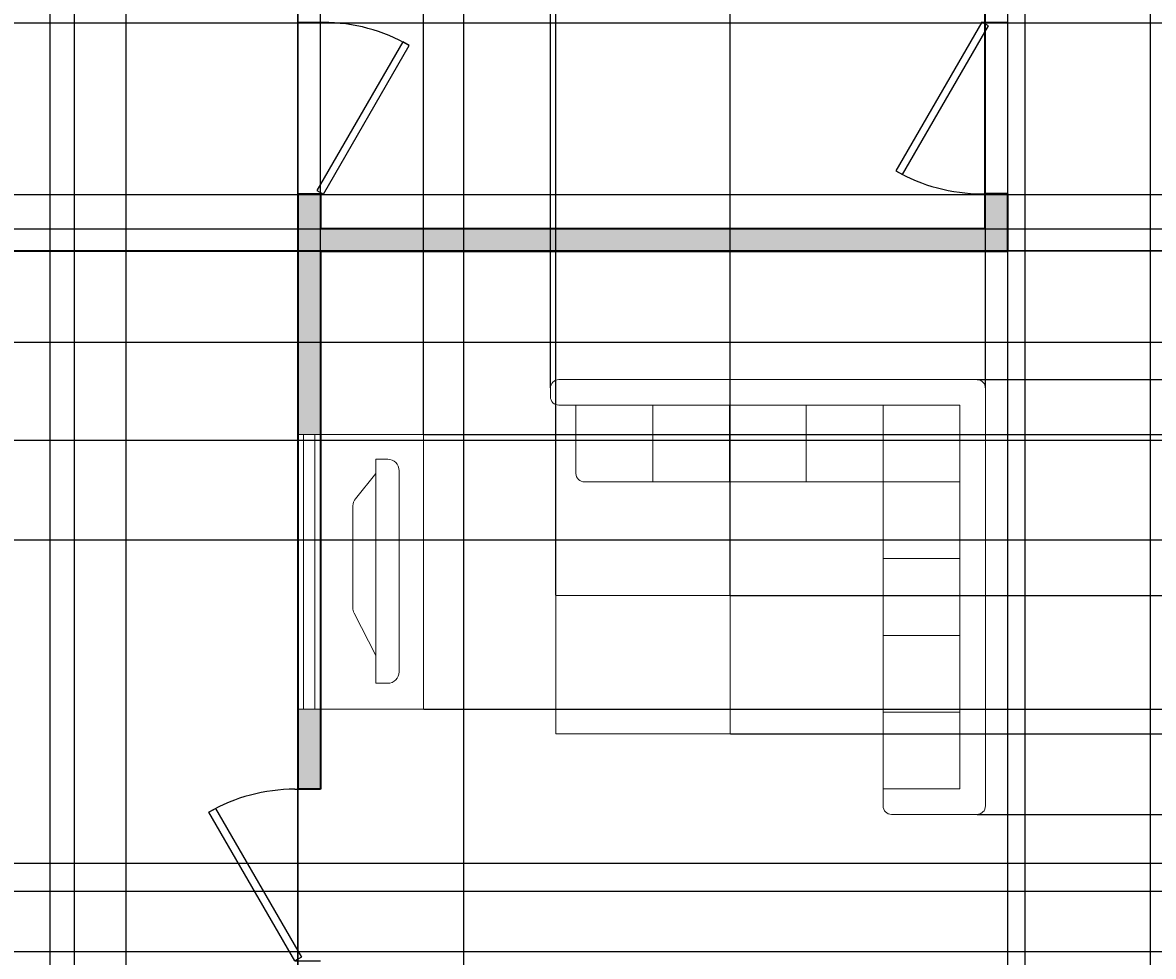
# Model space of a CAD drawing. Units: inches. Extents: x 1531 to 2263, y 2711 to 3216.
# Tile 5 of 12: x 1728 to 1925, y 2903 to 3066. Entities that reach past the tile are written whole.
import ezdxf

# ---------------------------------------------------------------- set-up
doc = ezdxf.new("R2010")
doc.units = ezdxf.units.IN
for name, color, linetype, lineweight in [('A-ANNO-DIMS', 2, 'Continuous', 18), ('A-DOOR', 3, 'Continuous', 25), ('A-EQPM', 8, 'Continuous', 18), ('A-FLOR-CASE', 9, 'Continuous', 18), ('A-FURN', 8, 'Continuous', 18), ('A-GLAZ', 4, 'Continuous', 18), ('A-WALL', 7, 'Continuous', 35)]:
    doc.layers.add(name, color=color, linetype=linetype, lineweight=lineweight)
doc.layers.add('A-WALL-PATT', color=18, linetype='Continuous', lineweight=13, true_color=0x000000)
doc.styles.get("Standard").update_dxf_attribs({"font": 'arial.ttf'})
doc.dimstyles.get("Standard").update_dxf_attribs({"dimtxt": 0.18, "dimasz": 0.18, "dimexe": 0.18, "dimexo": 0.0625, "dimgap": 0.09, "dimtad": 0, "dimtih": 1, "dimtoh": 1, "dimdec": 4, "dimzin": 0, "dimdsep": 46, "dimtxsty": 'Standard', "dimcen": 0.09, "dimadec": 0, "dimazin": 0, "dimtfac": 1, "dimtdec": 4, "dimtofl": 0, "dimtmove": 0, "dimatfit": 3, "dimfxl": 1, "dimtolj": 1, "dimtzin": 0, "dimarcsym": 0})

# ---------------------------------------------------------------- blocks, each defined once
blk = doc.blocks.new('*U5')
for p, q in [((0, 0), (0, -6)), ((-40, 0), (-40, -6))]:
    blk.add_line(p, q)
blk.add_lwpolyline([(0, 0), (-34.64, 20), (-35.52, 18.48), (-0.88, -1.52)], close=True)
blk.add_arc((0, 0), 40, 150, 180)
blk = doc.blocks.new('*U6')
for p, q in [((0, 0), (0, 6)), ((40, 0), (40, 6))]:
    blk.add_line(p, q)
blk.add_lwpolyline([(0, 0), (34.64, -20), (35.52, -18.48), (0.87, 1.52)], close=True)
blk.add_arc((0, 0), 40, 330, 0)
blk = doc.blocks.new('*U4')
for p, q in [((-40, 0), (-40, 6)), ((0, 0), (0, 6))]:
    blk.add_line(p, q)
blk.add_lwpolyline([(0, 0), (-34.64, -20), (-35.52, -18.48), (-0.88, 1.52)], close=True)
blk.add_arc((0, 0), 40, 180, 210)
blk = doc.blocks.new('*D58')
at = {"layer": 'A-ANNO-DIMS', "color": 0, "lineweight": -2, "transparency": 16777216}
for p, q in [((1715.91, 3097.69), (1715.91, 2711.06)), ((1775.91, 3097.72), (1775.91, 2711.06)), ((1716.09, 2711.24), (1745.69, 2711.24)), ((1775.73, 2711.24), (1746.13, 2711.24))]:
    blk.add_line(p, q, dxfattribs=at)
at = {"layer": 'A-ANNO-DIMS', "color": 0, "transparency": 16777216}
for points in [[(1716.09, 2711.27), (1716.09, 2711.21), (1715.91, 2711.24)], [(1775.73, 2711.27), (1775.73, 2711.21), (1775.91, 2711.24)]]:
    blk.add_solid(points, dxfattribs=at)
at = {"layer": 'Defpoints', "color": 0, "transparency": 16777216}
for p in [(1715.91, 3097.75), (1775.91, 3097.78), (1775.91, 2711.24)]:
    blk.add_point(p, dxfattribs=at)
at = {"layer": 'A-ANNO-DIMS', "color": 0, "transparency": 16777216, "insert": (1745.91, 2711.24), "char_height": 0.18, "attachment_point": 5}
blk.add_mtext('\\A1;60', dxfattribs=at)
blk = doc.blocks.new('*D59')
at = {"layer": 'A-ANNO-DIMS', "color": 0, "lineweight": -2, "transparency": 16777216}
for p, q in [((1779.91, 3029.85), (1779.91, 3216.47)), ((1780.09, 3216.29), (1837.63, 3216.29)), ((1895.73, 3216.29), (1838.19, 3216.29)), ((1895.91, 3029.91), (1895.91, 3216.47))]:
    blk.add_line(p, q, dxfattribs=at)
at = {"layer": 'A-ANNO-DIMS', "color": 0, "transparency": 16777216}
for points in [[(1780.09, 3216.32), (1780.09, 3216.26), (1779.91, 3216.29)], [(1895.73, 3216.32), (1895.73, 3216.26), (1895.91, 3216.29)]]:
    blk.add_solid(points, dxfattribs=at)
at = {"layer": 'Defpoints', "color": 0, "transparency": 16777216}
for p in [(1895.91, 3216.29), (1895.91, 3029.85), (1779.91, 3029.79)]:
    blk.add_point(p, dxfattribs=at)
at = {"layer": 'A-ANNO-DIMS', "color": 0, "transparency": 16777216, "insert": (1837.91, 3216.29), "char_height": 0.18, "attachment_point": 5}
blk.add_mtext('\\A1;116', dxfattribs=at)
blk = doc.blocks.new('*D60')
at = {"layer": 'A-ANNO-DIMS', "color": 0, "lineweight": -2, "transparency": 16777216}
for p, q in [((1899.91, 3097.79), (1899.91, 2711.06)), ((1955.91, 3097.81), (1955.91, 2711.06)), ((1900.09, 2711.24), (1927.69, 2711.24)), ((1955.73, 2711.24), (1928.13, 2711.24))]:
    blk.add_line(p, q, dxfattribs=at)
at = {"layer": 'A-ANNO-DIMS', "color": 0, "transparency": 16777216}
for points in [[(1900.09, 2711.27), (1900.09, 2711.21), (1899.91, 2711.24)], [(1955.73, 2711.27), (1955.73, 2711.21), (1955.91, 2711.24)]]:
    blk.add_solid(points, dxfattribs=at)
at = {"layer": 'Defpoints', "color": 0, "transparency": 16777216}
for p in [(1899.91, 3097.85), (1955.91, 3097.88), (1955.91, 2711.24)]:
    blk.add_point(p, dxfattribs=at)
at = {"layer": 'A-ANNO-DIMS', "color": 0, "transparency": 16777216, "insert": (1927.91, 2711.24), "char_height": 0.18, "attachment_point": 5}
blk.add_mtext('\\A1;56', dxfattribs=at)
blk = doc.blocks.new('*D64')
at = {"layer": 'A-ANNO-DIMS', "color": 0, "lineweight": -2, "transparency": 16777216}
for p, q in [((1779.85, 3025.79), (1531.04, 3025.79)), ((1531.22, 3025.61), (1531.22, 2960.97)), ((1531.22, 2895.96), (1531.22, 2960.6)), ((1775.85, 2895.78), (1531.04, 2895.78))]:
    blk.add_line(p, q, dxfattribs=at)
at = {"layer": 'A-ANNO-DIMS', "color": 0, "transparency": 16777216}
for points in [[(1531.19, 3025.61), (1531.25, 3025.61), (1531.22, 3025.79)], [(1531.19, 2895.96), (1531.25, 2895.96), (1531.22, 2895.78)]]:
    blk.add_solid(points, dxfattribs=at)
at = {"layer": 'Defpoints', "color": 0, "transparency": 16777216}
for p in [(1779.91, 3025.79), (1531.22, 2895.78), (1775.91, 2895.78)]:
    blk.add_point(p, dxfattribs=at)
at = {"layer": 'A-ANNO-DIMS', "color": 0, "transparency": 16777216, "insert": (1531.22, 2960.78), "char_height": 0.18, "attachment_point": 5}
blk.add_mtext('\\A1;130', dxfattribs=at)
blk = doc.blocks.new('*D66')
at = {"layer": 'A-ANNO-DIMS', "color": 0, "lineweight": -2, "transparency": 16777216}
for p, q in [((1577.91, 2895.74), (1577.91, 3216.47)), ((1578.09, 3216.29), (1676.63, 3216.29)), ((1775.73, 3216.29), (1677.19, 3216.29)), ((1775.91, 2895.85), (1775.91, 3216.47))]:
    blk.add_line(p, q, dxfattribs=at)
at = {"layer": 'A-ANNO-DIMS', "color": 0, "transparency": 16777216}
for points in [[(1578.09, 3216.32), (1578.09, 3216.26), (1577.91, 3216.29)], [(1775.73, 3216.32), (1775.73, 3216.26), (1775.91, 3216.29)]]:
    blk.add_solid(points, dxfattribs=at)
at = {"layer": 'Defpoints', "color": 0, "transparency": 16777216}
for p in [(1775.91, 3216.29), (1577.91, 2895.68), (1775.91, 2895.78)]:
    blk.add_point(p, dxfattribs=at)
at = {"layer": 'A-ANNO-DIMS', "color": 0, "transparency": 16777216, "insert": (1676.91, 3216.29), "char_height": 0.18, "attachment_point": 5}
blk.add_mtext('\\A1;198', dxfattribs=at)
blk = doc.blocks.new('*D68')
at = {"layer": 'A-ANNO-DIMS', "color": 0, "lineweight": -2, "transparency": 16777216}
for p, q in [((1736.91, 2839.83), (1736.91, 3216.47)), ((1737.09, 3216.29), (1770.69, 3216.29)), ((1804.73, 3216.29), (1771.13, 3216.29)), ((1804.91, 2839.86), (1804.91, 3216.47))]:
    blk.add_line(p, q, dxfattribs=at)
at = {"layer": 'A-ANNO-DIMS', "color": 0, "transparency": 16777216}
for points in [[(1737.09, 3216.32), (1737.09, 3216.26), (1736.91, 3216.29)], [(1804.73, 3216.32), (1804.73, 3216.26), (1804.91, 3216.29)]]:
    blk.add_solid(points, dxfattribs=at)
at = {"layer": 'Defpoints', "color": 0, "transparency": 16777216}
for p in [(1804.91, 3216.29), (1736.91, 2839.76), (1804.91, 2839.8)]:
    blk.add_point(p, dxfattribs=at)
at = {"layer": 'A-ANNO-DIMS', "color": 0, "transparency": 16777216, "insert": (1770.91, 3216.29), "char_height": 0.18, "attachment_point": 5}
blk.add_mtext('\\A1;68', dxfattribs=at)
blk = doc.blocks.new('*D77')
at = {"layer": 'A-ANNO-DIMS', "color": 0, "lineweight": -2, "transparency": 16777216}
for p, q in [((2094.81, 2975.33), (1531.04, 2975.33)), ((1531.22, 2975.15), (1531.22, 2939.52)), ((1531.22, 2903.53), (1531.22, 2939.16)), ((2094.81, 2903.35), (1531.04, 2903.35))]:
    blk.add_line(p, q, dxfattribs=at)
at = {"layer": 'A-ANNO-DIMS', "color": 0, "transparency": 16777216}
for points in [[(1531.19, 2975.15), (1531.25, 2975.15), (1531.22, 2975.33)], [(1531.19, 2903.53), (1531.25, 2903.53), (1531.22, 2903.35)]]:
    blk.add_solid(points, dxfattribs=at)
at = {"layer": 'Defpoints', "color": 0, "transparency": 16777216}
for p in [(2094.87, 2975.33), (1531.22, 2903.35), (2094.87, 2903.35)]:
    blk.add_point(p, dxfattribs=at)
at = {"layer": 'A-ANNO-DIMS', "color": 0, "transparency": 16777216, "insert": (1531.22, 2939.34), "char_height": 0.18, "attachment_point": 5}
blk.add_mtext('\\A1;71.98', dxfattribs=at)
blk = doc.blocks.new('*D86')
at = {"layer": 'A-ANNO-DIMS', "color": 0, "lineweight": -2, "transparency": 16777216}
for p, q in [((1715.97, 3065.75), (2262.37, 3065.75)), ((2262.19, 3065.57), (2262.19, 3050.93)), ((2262.19, 3035.93), (2262.19, 3050.57)), ((1715.97, 3035.75), (2262.37, 3035.75))]:
    blk.add_line(p, q, dxfattribs=at)
at = {"layer": 'A-ANNO-DIMS', "color": 0, "transparency": 16777216}
for points in [[(2262.16, 3065.57), (2262.22, 3065.57), (2262.19, 3065.75)], [(2262.16, 3035.93), (2262.22, 3035.93), (2262.19, 3035.75)]]:
    blk.add_solid(points, dxfattribs=at)
at = {"layer": 'Defpoints', "color": 0, "transparency": 16777216}
for p in [(1715.91, 3065.75), (2262.19, 3065.75), (1715.91, 3035.75)]:
    blk.add_point(p, dxfattribs=at)
at = {"layer": 'A-ANNO-DIMS', "color": 0, "transparency": 16777216, "insert": (2262.19, 3050.75), "char_height": 0.18, "attachment_point": 5}
blk.add_mtext('\\A1;30', dxfattribs=at)
blk = doc.blocks.new('*D87')
at = {"layer": 'A-ANNO-DIMS', "color": 0, "lineweight": -2, "transparency": 16777216}
for p, q in [((1721.91, 3101.69), (1721.91, 2711.06)), ((1745.91, 3101.7), (1745.91, 2711.06)), ((1722.09, 2711.24), (1733.69, 2711.24)), ((1745.73, 2711.24), (1734.13, 2711.24))]:
    blk.add_line(p, q, dxfattribs=at)
at = {"layer": 'A-ANNO-DIMS', "color": 0, "transparency": 16777216}
for points in [[(1722.09, 2711.27), (1722.09, 2711.21), (1721.91, 2711.24)], [(1745.73, 2711.27), (1745.73, 2711.21), (1745.91, 2711.24)]]:
    blk.add_solid(points, dxfattribs=at)
at = {"layer": 'Defpoints', "color": 0, "transparency": 16777216}
for p in [(1721.91, 3101.75), (1745.91, 3101.77), (1745.91, 2711.24)]:
    blk.add_point(p, dxfattribs=at)
at = {"layer": 'A-ANNO-DIMS', "color": 0, "transparency": 16777216, "insert": (1733.91, 2711.24), "char_height": 0.18, "attachment_point": 5}
blk.add_mtext('\\A1;24', dxfattribs=at)
blk = doc.blocks.new('*D98')
at = {"layer": 'A-ANNO-DIMS', "color": 0, "lineweight": -2, "transparency": 16777216}
for p, q in [((1820.04, 3001.95), (1820.04, 3216.47)), ((1820.22, 3216.29), (1857.83, 3216.29)), ((1895.86, 3216.29), (1858.26, 3216.29)), ((1896.04, 3001.95), (1896.04, 3216.47))]:
    blk.add_line(p, q, dxfattribs=at)
at = {"layer": 'A-ANNO-DIMS', "color": 0, "transparency": 16777216}
for points in [[(1820.22, 3216.32), (1820.22, 3216.26), (1820.04, 3216.29)], [(1895.86, 3216.32), (1895.86, 3216.26), (1896.04, 3216.29)]]:
    blk.add_solid(points, dxfattribs=at)
at = {"layer": 'Defpoints', "color": 0, "transparency": 16777216}
for p in [(1896.04, 3216.29), (1820.04, 3001.89), (1896.04, 3001.89)]:
    blk.add_point(p, dxfattribs=at)
at = {"layer": 'A-ANNO-DIMS', "color": 0, "transparency": 16777216, "insert": (1858.04, 3216.29), "char_height": 0.18, "attachment_point": 5}
blk.add_mtext('\\A1;76', dxfattribs=at)
blk = doc.blocks.new('*D99')
at = {"layer": 'A-ANNO-DIMS', "color": 0, "lineweight": -2, "transparency": 16777216}
for p, q in [((1894.62, 3003.38), (2262.37, 3003.38)), ((2262.19, 3003.2), (2262.19, 2965.56)), ((2262.19, 2927.56), (2262.19, 2965.19)), ((1894.62, 2927.38), (2262.37, 2927.38))]:
    blk.add_line(p, q, dxfattribs=at)
at = {"layer": 'A-ANNO-DIMS', "color": 0, "transparency": 16777216}
for points in [[(2262.16, 3003.2), (2262.22, 3003.2), (2262.19, 3003.38)], [(2262.16, 2927.56), (2262.22, 2927.56), (2262.19, 2927.38)]]:
    blk.add_solid(points, dxfattribs=at)
at = {"layer": 'Defpoints', "color": 0, "transparency": 16777216}
for p in [(1894.55, 3003.38), (1894.55, 2927.38), (2262.19, 2927.38)]:
    blk.add_point(p, dxfattribs=at)
at = {"layer": 'A-ANNO-DIMS', "color": 0, "transparency": 16777216, "insert": (2262.19, 2965.38), "char_height": 0.18, "attachment_point": 5}
blk.add_mtext('\\A1;76', dxfattribs=at)
blk = doc.blocks.new('*D101')
at = {"layer": 'A-ANNO-DIMS', "color": 0, "lineweight": -2, "transparency": 16777216}
for p, q in [((2228.85, 2918.81), (1531.04, 2918.81)), ((1531.22, 2918.63), (1531.22, 2897.08)), ((1531.22, 2875.18), (1531.22, 2896.72)), ((2228.85, 2875), (1531.04, 2875))]:
    blk.add_line(p, q, dxfattribs=at)
at = {"layer": 'A-ANNO-DIMS', "color": 0, "transparency": 16777216}
for points in [[(1531.19, 2918.63), (1531.25, 2918.63), (1531.22, 2918.81)], [(1531.19, 2875.18), (1531.25, 2875.18), (1531.22, 2875)]]:
    blk.add_solid(points, dxfattribs=at)
at = {"layer": 'Defpoints', "color": 0, "transparency": 16777216}
for p in [(2228.91, 2918.81), (1531.22, 2875), (2228.91, 2875)]:
    blk.add_point(p, dxfattribs=at)
at = {"layer": 'A-ANNO-DIMS', "color": 0, "transparency": 16777216, "insert": (1531.22, 2896.9), "char_height": 0.18, "attachment_point": 5}
blk.add_mtext('\\A1;43.81', dxfattribs=at)
blk = doc.blocks.new('*D110')
at = {"layer": 'A-ANNO-DIMS', "color": 0, "lineweight": -2, "transparency": 16777216}
for p, q in [((1711.97, 3035.75), (2262.37, 3035.75)), ((2262.19, 3035.57), (2262.19, 3032.93)), ((2262.19, 3029.93), (2262.19, 3032.57)), ((1711.97, 3029.75), (2262.37, 3029.75))]:
    blk.add_line(p, q, dxfattribs=at)
at = {"layer": 'A-ANNO-DIMS', "color": 0, "transparency": 16777216}
for points in [[(2262.16, 3035.57), (2262.22, 3035.57), (2262.19, 3035.75)], [(2262.16, 3029.93), (2262.22, 3029.93), (2262.19, 3029.75)]]:
    blk.add_solid(points, dxfattribs=at)
at = {"layer": 'Defpoints', "color": 0, "transparency": 16777216}
for p in [(1711.91, 3035.75), (2262.19, 3035.75), (1711.91, 3029.75)]:
    blk.add_point(p, dxfattribs=at)
at = {"layer": 'A-ANNO-DIMS', "color": 0, "transparency": 16777216, "insert": (2262.19, 3032.75), "char_height": 0.18, "attachment_point": 5}
blk.add_mtext('\\A1;6', dxfattribs=at)
blk = doc.blocks.new('*D112')
at = {"layer": 'A-ANNO-DIMS', "color": 0, "lineweight": -2, "transparency": 16777216}
for p, q in [((1721.97, 3009.94), (2262.37, 3009.94)), ((2262.19, 3009.76), (2262.19, 2962.12)), ((2262.19, 2914.12), (2262.19, 2961.76)), ((1721.97, 2913.94), (2262.37, 2913.94))]:
    blk.add_line(p, q, dxfattribs=at)
at = {"layer": 'A-ANNO-DIMS', "color": 0, "transparency": 16777216}
for points in [[(2262.16, 3009.76), (2262.22, 3009.76), (2262.19, 3009.94)], [(2262.16, 2914.12), (2262.22, 2914.12), (2262.19, 2913.94)]]:
    blk.add_solid(points, dxfattribs=at)
at = {"layer": 'Defpoints', "color": 0, "transparency": 16777216}
for p in [(1721.91, 3009.94), (1721.91, 2913.94), (2262.19, 2913.94)]:
    blk.add_point(p, dxfattribs=at)
at = {"layer": 'A-ANNO-DIMS', "color": 0, "transparency": 16777216, "insert": (2262.19, 2961.94), "char_height": 0.18, "attachment_point": 5}
blk.add_mtext('\\A1;96', dxfattribs=at)
blk = doc.blocks.new('*D114')
at = {"layer": 'A-ANNO-DIMS', "color": 0, "lineweight": -2, "transparency": 16777216}
for p, q in [((1577.97, 2913.94), (2262.37, 2913.94)), ((2262.19, 2913.76), (2262.19, 2904.99)), ((2262.19, 2895.86), (2262.19, 2904.63)), ((1577.97, 2895.68), (2262.37, 2895.68))]:
    blk.add_line(p, q, dxfattribs=at)
at = {"layer": 'A-ANNO-DIMS', "color": 0, "transparency": 16777216}
for points in [[(2262.16, 2913.76), (2262.22, 2913.76), (2262.19, 2913.94)], [(2262.16, 2895.86), (2262.22, 2895.86), (2262.19, 2895.68)]]:
    blk.add_solid(points, dxfattribs=at)
at = {"layer": 'Defpoints', "color": 0, "transparency": 16777216}
for p in [(1577.91, 2913.94), (1577.91, 2895.68), (2262.19, 2895.68)]:
    blk.add_point(p, dxfattribs=at)
at = {"layer": 'A-ANNO-DIMS', "color": 0, "transparency": 16777216, "insert": (2262.19, 2904.81), "char_height": 0.18, "attachment_point": 5}
blk.add_mtext('\\A1;18.26', dxfattribs=at)
blk = doc.blocks.new('*D115')
at = {"layer": 'A-ANNO-DIMS', "color": 0, "lineweight": -2, "transparency": 16777216}
for p, q in [((1779.91, 2993.83), (1779.91, 3216.47)), ((1780.09, 3216.29), (1799.58, 3216.29)), ((1819.86, 3216.29), (1800.37, 3216.29)), ((1820.04, 3001.95), (1820.04, 3216.47))]:
    blk.add_line(p, q, dxfattribs=at)
at = {"layer": 'A-ANNO-DIMS', "color": 0, "transparency": 16777216}
for points in [[(1780.09, 3216.32), (1780.09, 3216.26), (1779.91, 3216.29)], [(1819.86, 3216.32), (1819.86, 3216.26), (1820.04, 3216.29)]]:
    blk.add_solid(points, dxfattribs=at)
at = {"layer": 'Defpoints', "color": 0, "transparency": 16777216}
for p in [(1820.04, 3216.29), (1820.04, 3001.89), (1779.91, 2993.76)]:
    blk.add_point(p, dxfattribs=at)
at = {"layer": 'A-ANNO-DIMS', "color": 0, "transparency": 16777216, "insert": (1799.98, 3216.29), "char_height": 0.18, "attachment_point": 5}
blk.add_mtext('\\A1;40.13', dxfattribs=at)
blk = doc.blocks.new('*D116')
at = {"layer": 'A-ANNO-DIMS', "color": 0, "lineweight": -2, "transparency": 16777216}
for p, q in [((1899.97, 3025.85), (2262.37, 3025.85)), ((2262.19, 3025.67), (2262.19, 3014.79)), ((2262.19, 3003.56), (2262.19, 3014.43)), ((1894.62, 3003.38), (2262.37, 3003.38))]:
    blk.add_line(p, q, dxfattribs=at)
at = {"layer": 'A-ANNO-DIMS', "color": 0, "transparency": 16777216}
for points in [[(2262.16, 3025.67), (2262.22, 3025.67), (2262.19, 3025.85)], [(2262.16, 3003.56), (2262.22, 3003.56), (2262.19, 3003.38)]]:
    blk.add_solid(points, dxfattribs=at)
at = {"layer": 'Defpoints', "color": 0, "transparency": 16777216}
for p in [(1899.91, 3025.85), (1894.55, 3003.38), (2262.19, 3003.38)]:
    blk.add_point(p, dxfattribs=at)
at = {"layer": 'A-ANNO-DIMS', "color": 0, "transparency": 16777216, "insert": (2262.19, 3014.61), "char_height": 0.18, "attachment_point": 5}
blk.add_mtext('\\A1;22.47', dxfattribs=at)
blk = doc.blocks.new('*D117')
at = {"layer": 'A-ANNO-DIMS', "color": 0, "lineweight": -2, "transparency": 16777216}
for p, q in [((1821.02, 2965.7), (1821.02, 3216.47)), ((1821.2, 3216.29), (1835.77, 3216.29)), ((1851.26, 3216.29), (1836.69, 3216.29)), ((1851.44, 2965.7), (1851.44, 3216.47))]:
    blk.add_line(p, q, dxfattribs=at)
at = {"layer": 'A-ANNO-DIMS', "color": 0, "transparency": 16777216}
for points in [[(1821.2, 3216.32), (1821.2, 3216.26), (1821.02, 3216.29)], [(1851.26, 3216.32), (1851.26, 3216.26), (1851.44, 3216.29)]]:
    blk.add_solid(points, dxfattribs=at)
at = {"layer": 'Defpoints', "color": 0, "transparency": 16777216}
for p in [(1851.44, 3216.29), (1821.02, 2965.63), (1851.44, 2965.63)]:
    blk.add_point(p, dxfattribs=at)
at = {"layer": 'A-ANNO-DIMS', "color": 0, "transparency": 16777216, "insert": (1836.23, 3216.29), "char_height": 0.18, "attachment_point": 5}
blk.add_mtext('\\A1;30.417', dxfattribs=at)
blk = doc.blocks.new('*D118')
at = {"layer": 'A-ANNO-DIMS', "color": 0, "lineweight": -2, "transparency": 16777216}
for p, q in [((1851.5, 2965.63), (2262.37, 2965.63)), ((2262.19, 2965.45), (2262.19, 2953.74)), ((2262.19, 2941.67), (2262.19, 2953.38)), ((1851.5, 2941.49), (2262.37, 2941.49))]:
    blk.add_line(p, q, dxfattribs=at)
at = {"layer": 'A-ANNO-DIMS', "color": 0, "transparency": 16777216}
for points in [[(2262.16, 2965.45), (2262.22, 2965.45), (2262.19, 2965.63)], [(2262.16, 2941.67), (2262.22, 2941.67), (2262.19, 2941.49)]]:
    blk.add_solid(points, dxfattribs=at)
at = {"layer": 'Defpoints', "color": 0, "transparency": 16777216}
for p in [(1851.44, 2965.63), (1851.44, 2941.49), (2262.19, 2941.49)]:
    blk.add_point(p, dxfattribs=at)
at = {"layer": 'A-ANNO-DIMS', "color": 0, "transparency": 16777216, "insert": (2262.19, 2953.56), "char_height": 0.18, "attachment_point": 5}
blk.add_mtext('\\A1;24.14', dxfattribs=at)
blk = doc.blocks.new('*D119')
at = {"layer": 'A-ANNO-DIMS', "color": 0, "lineweight": -2, "transparency": 16777216}
for p, q in [((1779.91, 2993.83), (1779.91, 3216.47)), ((1780.09, 3216.29), (1788.7, 3216.29)), ((1797.73, 3216.29), (1789.12, 3216.29)), ((1797.91, 2993.83), (1797.91, 3216.47))]:
    blk.add_line(p, q, dxfattribs=at)
at = {"layer": 'A-ANNO-DIMS', "color": 0, "transparency": 16777216}
for points in [[(1780.09, 3216.32), (1780.09, 3216.26), (1779.91, 3216.29)], [(1797.73, 3216.32), (1797.73, 3216.26), (1797.91, 3216.29)]]:
    blk.add_solid(points, dxfattribs=at)
at = {"layer": 'Defpoints', "color": 0, "transparency": 16777216}
for p in [(1797.91, 3216.29), (1779.91, 2993.76), (1797.91, 2993.76)]:
    blk.add_point(p, dxfattribs=at)
at = {"layer": 'A-ANNO-DIMS', "color": 0, "transparency": 16777216, "insert": (1788.91, 3216.29), "char_height": 0.18, "attachment_point": 5}
blk.add_mtext('\\A1;18', dxfattribs=at)
blk = doc.blocks.new('*D120')
at = {"layer": 'A-ANNO-DIMS', "color": 0, "lineweight": -2, "transparency": 16777216}
for p, q in [((1797.97, 2993.76), (2262.37, 2993.76)), ((2262.19, 2993.58), (2262.19, 2969.95)), ((2262.19, 2945.94), (2262.19, 2969.58)), ((1797.97, 2945.76), (2262.37, 2945.76))]:
    blk.add_line(p, q, dxfattribs=at)
at = {"layer": 'A-ANNO-DIMS', "color": 0, "transparency": 16777216}
for points in [[(2262.16, 2993.58), (2262.22, 2993.58), (2262.19, 2993.76)], [(2262.16, 2945.94), (2262.22, 2945.94), (2262.19, 2945.76)]]:
    blk.add_solid(points, dxfattribs=at)
at = {"layer": 'Defpoints', "color": 0, "transparency": 16777216}
for p in [(1797.91, 2993.76), (2262.19, 2993.76), (1797.91, 2945.76)]:
    blk.add_point(p, dxfattribs=at)
at = {"layer": 'A-ANNO-DIMS', "color": 0, "transparency": 16777216, "insert": (2262.19, 2969.76), "char_height": 0.18, "attachment_point": 5}
blk.add_mtext('\\A1;48', dxfattribs=at)
blk = doc.blocks.new('*D122')
at = {"layer": 'A-ANNO-DIMS', "color": 0, "lineweight": -2, "transparency": 16777216}
for p, q in [((1955.85, 3025.88), (1531.04, 3025.88)), ((1531.22, 3025.7), (1531.22, 3009.49)), ((1531.22, 2992.91), (1531.22, 3009.12)), ((1968.31, 2992.73), (1531.04, 2992.73))]:
    blk.add_line(p, q, dxfattribs=at)
at = {"layer": 'A-ANNO-DIMS', "color": 0, "transparency": 16777216}
for points in [[(1531.19, 3025.7), (1531.25, 3025.7), (1531.22, 3025.88)], [(1531.19, 2992.91), (1531.25, 2992.91), (1531.22, 2992.73)]]:
    blk.add_solid(points, dxfattribs=at)
at = {"layer": 'Defpoints', "color": 0, "transparency": 16777216}
for p in [(1531.22, 3025.88), (1955.91, 3025.88), (1968.37, 2992.73)]:
    blk.add_point(p, dxfattribs=at)
at = {"layer": 'A-ANNO-DIMS', "color": 0, "transparency": 16777216, "insert": (1531.22, 3009.3), "char_height": 0.18, "attachment_point": 5}
blk.add_mtext('\\A1;33.146', dxfattribs=at)
blk = doc.blocks.new('*D126')
at = {"layer": 'A-ANNO-DIMS', "color": 0, "lineweight": -2, "transparency": 16777216}
for p, q in [((1902.99, 2850), (1902.99, 3216.47)), ((1903.17, 3216.29), (1913.45, 3216.29)), ((1924.67, 3216.29), (1914.38, 3216.29)), ((1924.85, 2850), (1924.85, 3216.47))]:
    blk.add_line(p, q, dxfattribs=at)
at = {"layer": 'A-ANNO-DIMS', "color": 0, "transparency": 16777216}
for points in [[(1903.17, 3216.32), (1903.17, 3216.26), (1902.99, 3216.29)], [(1924.67, 3216.32), (1924.67, 3216.26), (1924.85, 3216.29)]]:
    blk.add_solid(points, dxfattribs=at)
at = {"layer": 'Defpoints', "color": 0, "transparency": 16777216}
for p in [(1924.85, 3216.29), (1902.99, 2849.94), (1924.85, 2849.94)]:
    blk.add_point(p, dxfattribs=at)
at = {"layer": 'A-ANNO-DIMS', "color": 0, "transparency": 16777216, "insert": (1913.92, 3216.29), "char_height": 0.18, "attachment_point": 5}
blk.add_mtext('\\A1;21.866', dxfattribs=at)
blk = doc.blocks.new('*D128')
at = {"layer": 'A-ANNO-DIMS', "color": 0, "lineweight": -2, "transparency": 16777216}
for p, q in [((1710.84, 2841.9), (1710.84, 3216.47)), ((1711.02, 3216.29), (1721.3, 3216.29)), ((1732.52, 3216.29), (1722.23, 3216.29)), ((1732.7, 2841.9), (1732.7, 3216.47))]:
    blk.add_line(p, q, dxfattribs=at)
at = {"layer": 'A-ANNO-DIMS', "color": 0, "transparency": 16777216}
for points in [[(1711.02, 3216.32), (1711.02, 3216.26), (1710.84, 3216.29)], [(1732.52, 3216.32), (1732.52, 3216.26), (1732.7, 3216.29)]]:
    blk.add_solid(points, dxfattribs=at)
at = {"layer": 'Defpoints', "color": 0, "transparency": 16777216}
for p in [(1732.7, 3216.29), (1710.84, 2841.84), (1732.7, 2841.84)]:
    blk.add_point(p, dxfattribs=at)
at = {"layer": 'A-ANNO-DIMS', "color": 0, "transparency": 16777216, "insert": (1721.77, 3216.29), "char_height": 0.18, "attachment_point": 5}
blk.add_mtext('\\A1;21.866', dxfattribs=at)

msp = doc.modelspace()

# ---------------------------------------------------------------- hatches: boundary and pattern name
at = {"layer": 'A-WALL-PATT'}
h = msp.add_hatch(color=256, dxfattribs=at)
h.dxf.hatch_style = 1
h.paths.add_polyline_path([(1899.9101, 3035.8479), (1895.9101, 3035.8458), (1895.9101, 3029.8458), (1779.9101, 3029.7852), (1779.9101, 3035.7831), (1775.9101, 3035.7831), (1775.9101, 2993.7637), (1779.9101, 2993.7637), (1779.9101, 3025.7852), (1899.9101, 3025.8479)])
h = msp.add_hatch(color=256, dxfattribs=at)
h.dxf.hatch_style = 1
h.paths.add_polyline_path([(1779.9101, 2945.7637), (1775.9101, 2945.7637), (1775.9101, 2931.7831), (1779.9101, 2931.7852)])

# ---------------------------------------------------------------- linework, layer by layer
at = {"layer": 'A-EQPM'}
msp.add_lwpolyline([(1791.628, 2989.4482), (1789.589, 2989.4482), (1789.589, 2950.2998), (1791.628, 2950.2998, 0.41421356), (1793.628, 2952.2998), (1793.628, 2987.4482, 0.41421356)], format="xyb", close=True, dxfattribs=at)
msp.add_lwpolyline([(1789.589, 2986.9555), (1786.0009, 2982.5618, 0.17289395), (1785.55, 2981.2967), (1785.55, 2963.4948, 0.11893715), (1785.7701, 2962.5827), (1789.589, 2955.1298)], format="xyb", dxfattribs=at)
msp.add_lwpolyline([(1789.589, 2952.9285), (1789.589, 2984.7542)], dxfattribs=at)
at = {"layer": 'A-FLOR-CASE'}
msp.add_lwpolyline([(1779.9101, 2993.7637), (1797.9101, 2993.7637), (1797.9101, 2945.7637), (1779.9101, 2945.7637)], close=True, dxfattribs=at)
at = {"layer": 'A-FURN'}
for p, q in [((1821.5336, 3003.376), (1894.5532, 3003.376)), ((1820.0434, 3001.8858), (1820.0434, 3000.3956)), ((1896.0434, 3001.8858), (1896.0434, 2928.8661)), ((1821.5336, 2998.9054), (1891.5728, 2998.9054)), ((1891.5728, 2998.9054), (1891.5728, 2931.8465)), ((1891.5728, 2931.8465), (1878.161, 2931.8465)), ((1878.161, 2931.8465), (1878.161, 2928.8661)), ((1894.5532, 2927.376), (1879.6512, 2927.376))]:
    msp.add_line(p, q, dxfattribs=at)
msp.add_lwpolyline([(1837.9257, 2998.9054), (1824.514, 2998.9054), (1824.514, 2986.9838, 0.41421356), (1826.0042, 2985.4936), (1837.9257, 2985.4936)], format="xyb", close=True, dxfattribs=at)
for points in [[(1851.3375, 2998.9054), (1837.9257, 2998.9054), (1837.9257, 2985.4936), (1851.3375, 2985.4936)], [(1864.7493, 2998.9054), (1851.3375, 2998.9054), (1851.3375, 2985.4936), (1864.7493, 2985.4936)], [(1878.161, 2998.9054), (1864.7493, 2998.9054), (1864.7493, 2985.4936), (1878.161, 2985.4936)], [(1891.5728, 2998.9054), (1878.161, 2998.9054), (1878.161, 2985.4936), (1891.5728, 2985.4936)], [(1891.5728, 2985.4936), (1878.161, 2985.4936), (1878.161, 2972.0818), (1891.5728, 2972.0818)], [(1891.5728, 2972.0818), (1878.161, 2972.0818), (1878.161, 2958.6701), (1891.5728, 2958.6701)], [(1821.0226, 2965.6329), (1851.4391, 2965.6329), (1851.4391, 2941.4913), (1821.0226, 2941.4913)], [(1891.5728, 2958.6701), (1878.161, 2958.6701), (1878.161, 2945.2583), (1891.5728, 2945.2583)], [(1891.5728, 2945.2583), (1878.161, 2945.2583), (1878.161, 2931.8465), (1891.5728, 2931.8465)]]:
    msp.add_lwpolyline(points, close=True, dxfattribs=at)
for centre, start, end in [((1821.5336, 3001.8858), 90, 180), ((1894.5532, 3001.8858), 0, 90), ((1821.5336, 3000.3956), 180, 270), ((1879.6512, 2928.8661), 180, 270), ((1894.5532, 2928.8661), 270, 0)]:
    msp.add_arc(centre, 1.4902, start, end, dxfattribs=at)
at = {"layer": 'A-GLAZ'}
for p, q in [((1776.9101, 2945.7637), (1776.9101, 2993.7637)), ((1778.9101, 2945.7637), (1778.9101, 2993.7637))]:
    msp.add_line(p, q, dxfattribs=at)
for points in [[(1779.9101, 2993.7637), (1775.9101, 2993.7637)], [(1775.9101, 2945.7637), (1779.9101, 2945.7637)]]:
    msp.add_lwpolyline(points, dxfattribs=at)
at = {"layer": 'A-WALL'}
for p, q in [((1779.9101, 3035.7852), (1775.907, 3035.7831)), ((1775.9101, 3035.7831), (1775.9101, 2931.7831)), ((1779.9101, 3035.7852), (1779.9101, 3029.7852)), ((1899.9101, 3035.8479), (1895.907, 3035.8458)), ((1895.9101, 3035.8458), (1895.9101, 3029.8458)), ((1899.9101, 3035.8479), (1899.9101, 3025.8479)), ((1779.9101, 3029.7852), (1895.9101, 3029.8458)), ((1779.9101, 3025.7852), (1899.9101, 3025.8479)), ((1779.9101, 3025.7852), (1779.9101, 2931.7852)), ((1779.9101, 2931.7852), (1775.8913, 2931.7831))]:
    msp.add_line(p, q, dxfattribs=at)

# ---------------------------------------------------------------- block references
at = {"layer": 'A-DOOR', "xscale": 0.75, "yscale": 0.75, "zscale": 0.75, "rotation": 270}
for name, p in [('*U5', (1780.3913, 3035.7831)), ('*U6', (1895.4101, 3065.8479)), ('*U4', (1775.4101, 2901.7852))]:
    msp.add_blockref(name, p, dxfattribs=at)

# ---------------------------------------------------------------- dimensions: what is measured, and where the dimension line sits
at = {"layer": 'A-ANNO-DIMS'}
for base, p1, p2, override, picture, middle in [((1775.9101, 3216.295), (1577.9111, 2895.6796), (1775.9101, 2895.7831), {"dimdec": 0, "dimlfac": 1, "dimrnd": 0, "dimzin": 0, "dimdsep": 46, "dimlunit": 2}, '*D66', (1676.9106, 3216.295)), ((1732.7021, 3216.295), (1710.8363, 2841.8359), (1732.7021, 2841.8359), {"dimdec": 3, "dimlfac": 1, "dimrnd": 0, "dimzin": 0, "dimdsep": 46, "dimlunit": 2}, '*D128', (1721.7692, 3216.295)), ((1804.9101, 3216.295), (1736.9101, 2839.7627), (1804.9101, 2839.7983), {"dimdec": 0, "dimlfac": 1, "dimrnd": 0, "dimzin": 0, "dimdsep": 46, "dimlunit": 2}, '*D68', (1770.9101, 3216.295)), ((1895.9101, 3216.295), (1779.9101, 3029.7852), (1895.9101, 3029.8458), {"dimdec": 0, "dimlfac": 1, "dimrnd": 0, "dimzin": 0, "dimdsep": 46, "dimlunit": 2}, '*D59', (1837.9101, 3216.295)), ((1820.0434, 3216.295), (1779.9101, 2993.7637), (1820.0434, 3001.8858), {"dimdec": 2, "dimlfac": 1, "dimrnd": 0, "dimzin": 0, "dimdsep": 46, "dimlunit": 2}, '*D115', (1799.9768, 3216.295)), ((1797.9101, 3216.295), (1779.9101, 2993.7637), (1797.9101, 2993.7637), {"dimdec": 0, "dimlfac": 1, "dimrnd": 0, "dimzin": 0, "dimdsep": 46, "dimlunit": 2}, '*D119', (1788.9101, 3216.295)), ((1896.0434, 3216.295), (1820.0434, 3001.8858), (1896.0434, 3001.8858), {"dimdec": 0, "dimlfac": 1, "dimrnd": 0, "dimzin": 0, "dimdsep": 46, "dimlunit": 2}, '*D98', (1858.0434, 3216.295)), ((1851.43908, 3216.295), (1821.02257, 2965.63292), (1851.43908, 2965.63292), {"dimdec": 3, "dimlfac": 1, "dimrnd": 0, "dimzin": 0, "dimdsep": 46, "dimlunit": 2}, '*D117', (1836.23083, 3216.295)), ((1924.852, 3216.295), (1902.9862, 2849.9364), (1924.852, 2849.9364), {"dimdec": 3, "dimlfac": 1, "dimrnd": 0, "dimzin": 0, "dimdsep": 46, "dimlunit": 2}, '*D126', (1913.9191, 3216.295)), ((1745.9101, 2711.2407), (1721.9101, 3101.7549), (1745.9101, 3101.7674), {"dimdec": 0, "dimlfac": 1, "dimrnd": 0, "dimzin": 0, "dimdsep": 46, "dimlunit": 2}, '*D87', (1733.9101, 2711.2407)), ((1775.9101, 2711.2407), (1715.9101, 3097.7517), (1775.9101, 3097.7831), {"dimdec": 0, "dimlfac": 1, "dimrnd": 0, "dimzin": 0, "dimdsep": 46, "dimlunit": 2}, '*D58', (1745.9101, 2711.2407)), ((1955.9101, 2711.2407), (1899.9101, 3097.8479), (1955.9101, 3097.8772), {"dimdec": 0, "dimlfac": 1, "dimrnd": 0, "dimzin": 0, "dimdsep": 46, "dimlunit": 2}, '*D60', (1927.9101, 2711.2407))]:
    dim = msp.add_linear_dim(base=base, p1=p1, p2=p2, dimstyle='Standard', override=override, dxfattribs=at)
    dim.commit()
    dim.dimension.update_dxf_attribs({"geometry": picture, "text_midpoint": middle})
for base, p1, p2, override, picture, middle in [((2262.1851, 3065.7517), (1715.9101, 3035.7517), (1715.9101, 3065.7517), {"dimdec": 0, "dimlfac": 1, "dimrnd": 0, "dimzin": 0, "dimdsep": 46, "dimlunit": 2}, '*D86', (2262.1851, 3050.7517)), ((2262.1851, 3035.7496), (1711.9101, 3029.7496), (1711.9101, 3035.7496), {"dimdec": 0, "dimlfac": 1, "dimrnd": 0, "dimzin": 0, "dimdsep": 46, "dimlunit": 2}, '*D110', (2262.1851, 3032.7496)), ((1531.2212, 3025.8772), (1968.3722, 2992.7314), (1955.9101, 3025.8772), {"dimdec": 3, "dimlfac": 1, "dimrnd": 0, "dimzin": 0, "dimdsep": 46, "dimlunit": 2}, '*D122', (1531.2212, 3009.3043)), ((1531.2212, 2895.7831), (1779.9101, 3025.7852), (1775.9101, 2895.7831), {"dimdec": 0, "dimlfac": 1, "dimrnd": 0, "dimzin": 0, "dimdsep": 46, "dimlunit": 2}, '*D64', (1531.2212, 2960.7841)), ((2262.1851, 3003.376), (1899.9101, 3025.8479), (1894.5532, 3003.376), {"dimdec": 2, "dimlfac": 1, "dimrnd": 0, "dimzin": 0, "dimdsep": 46, "dimlunit": 2}, '*D116', (2262.1851, 3014.6119)), ((2262.1851, 2913.9378), (1721.9111, 3009.9378), (1721.9111, 2913.9378), {"dimdec": 0, "dimlfac": 1, "dimrnd": 0, "dimzin": 0, "dimdsep": 46, "dimlunit": 2}, '*D112', (2262.1851, 2961.9378)), ((2262.1851, 2927.376), (1894.5532, 3003.376), (1894.5532, 2927.376), {"dimdec": 0, "dimlfac": 1, "dimrnd": 0, "dimzin": 0, "dimdsep": 46, "dimlunit": 2}, '*D99', (2262.1851, 2965.376)), ((2262.1851, 2993.7637), (1797.9101, 2945.7637), (1797.9101, 2993.7637), {"dimdec": 0, "dimlfac": 1, "dimrnd": 0, "dimzin": 0, "dimdsep": 46, "dimlunit": 2}, '*D120', (2262.1851, 2969.7637)), ((1531.2212, 2903.3482), (2094.8725, 2975.3315), (2094.8725, 2903.3482), {"dimdec": 2, "dimlfac": 1, "dimrnd": 0, "dimzin": 0, "dimdsep": 46, "dimlunit": 2}, '*D77', (1531.2212, 2939.3398)), ((2262.1851, 2941.4913), (1851.4391, 2965.6329), (1851.4391, 2941.4913), {"dimdec": 2, "dimlfac": 1, "dimrnd": 0, "dimzin": 0, "dimdsep": 46, "dimlunit": 2}, '*D118', (2262.1851, 2953.5621)), ((1531.2212, 2874.9957), (2228.9101, 2918.8056), (2228.9101, 2874.9957), {"dimdec": 2, "dimlfac": 1, "dimrnd": 0, "dimzin": 0, "dimdsep": 46, "dimlunit": 2}, '*D101', (1531.2212, 2896.9007)), ((2262.1851, 2895.6796), (1577.9111, 2913.9378), (1577.9111, 2895.6796), {"dimdec": 2, "dimlfac": 1, "dimrnd": 0, "dimzin": 0, "dimdsep": 46, "dimlunit": 2}, '*D114', (2262.1851, 2904.8087))]:
    dim = msp.add_linear_dim(base=base, p1=p1, p2=p2, angle=90, dimstyle='Standard', override=override, dxfattribs=at)
    dim.commit()
    dim.dimension.update_dxf_attribs({"geometry": picture, "text_midpoint": middle})

doc.saveas('drawing.dxf')
